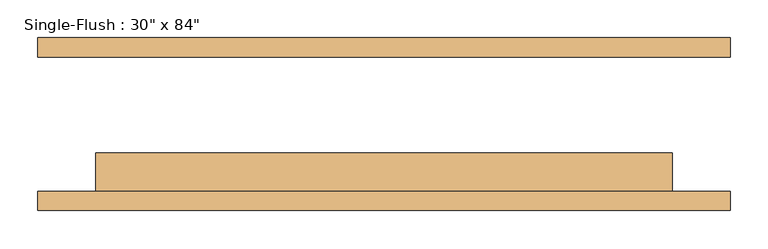
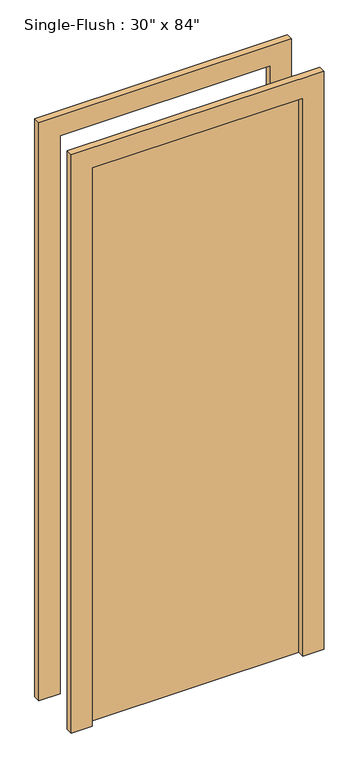
"""IFC4 building model written with IfcOpenShell, lengths in millimetres: door geometry."""

from ifc_helpers import new_model, si_unit, frame, origin, origin_with_axes, place, context, project, spatial, polyline, outline, extrude, source, transform, mapped, element, save


def door_b1104dde(model_context):
    return source(origin(), model_context, "Body", "SweptSolid", [
        extrude(outline(polyline([(2209.8, -457.2), (0.0, -457.2), (0.0, -381.0), (2133.6, -381.0), (2133.6, 381.0), (0.0, 381.0), (0.0, 457.2), (2209.8, 457.2), (2209.8, -457.2)])), frame((0.0, -114.3, 0.0), z_axis=(0.0, 1.0, 0.0), x_axis=(0.0, 0.0, 1.0)), (0.0, 0.0, 1.0), 25.4),
        extrude(outline(polyline([(2209.8, 457.2), (2209.8, -457.2), (0.0, -457.2), (0.0, -381.0), (2133.6, -381.0), (2133.6, 381.0), (0.0, 381.0), (0.0, 457.2), (2209.8, 457.2)])), frame((0.0, 88.9, 0.0), z_axis=(0.0, 1.0, 0.0), x_axis=(0.0, 0.0, 1.0)), (0.0, 0.0, 1.0), 25.4),
        extrude(outline(polyline([(381.0, -38.1), (381.0, -88.9), (-381.0, -88.9), (-381.0, -38.1), (381.0, -38.1)])), origin_with_axes(), (0.0, 0.0, 1.0), 2133.6),
    ])


if __name__ == "__main__":
    model = new_model("IFC4")
    model_context = context("Model", 3, world=origin())
    ifc_project = project(units=[si_unit("LENGTHUNIT", "METRE", prefix="MILLI")], contexts=[model_context])
    site = spatial("IfcSite", under=ifc_project)
    building = spatial("IfcBuilding", under=site)
    placement = place(None, origin())
    door_shape = door_b1104dde(model_context)
    element("IfcDoor", 1, ObjectType="Single-Flush : 30\" x 84\"", at=placement, inside=building, context=model_context, shape_type="MappedRepresentation", body=[
        mapped(door_shape, transform((0.0, 0.0, 0.0), x_axis=(1.0, 0.0, 0.0), y_axis=(0.0, 1.0, 0.0), z_axis=(0.0, 0.0, 1.0))),
    ])
    save(model, "model.ifc")

# Revit data of these elements
# Type "Single-Flush : 30\" x 84\""
#   Type Mark = "4"
#   Construction Type Id = "MDOOR"
#   Assembly Code = "C1020"
#   Analytic Construction = "Metal"
#   Thickness = 0' - 2"
#   Heat Transfer Coefficient (U) = 0.651978 BTU/(h·ft²·°F)
#   Height = 7' - 0"
#   Trim Projection Ext = 0' - 1"
#   Trim Projection Int = 0' - 1"
#   Trim Width = 0' - 3"
#   Width = 2' - 6"
#   Define Thermal Properties by = 1
#   Door Material = Door - Panel
#   Frame Material = Door - Frame
#   Visual Light Transmittance = 0
#   Solar Heat Gain Coefficient = 0
#   Function = (empty or 0)
#   Wall Closure = (empty or 0)
# Element 1 (IfcDoor, "Single-Flush : 30\" x 84\"")
#   Materials on its faces: "Door - Frame", "Door - Panel"
# Materials
#   "Door - Panel": class "Wood", colour RGB 210 159 95, transparency 0
#   "Door - Frame": colour RGB 118 70 51, transparency 0
